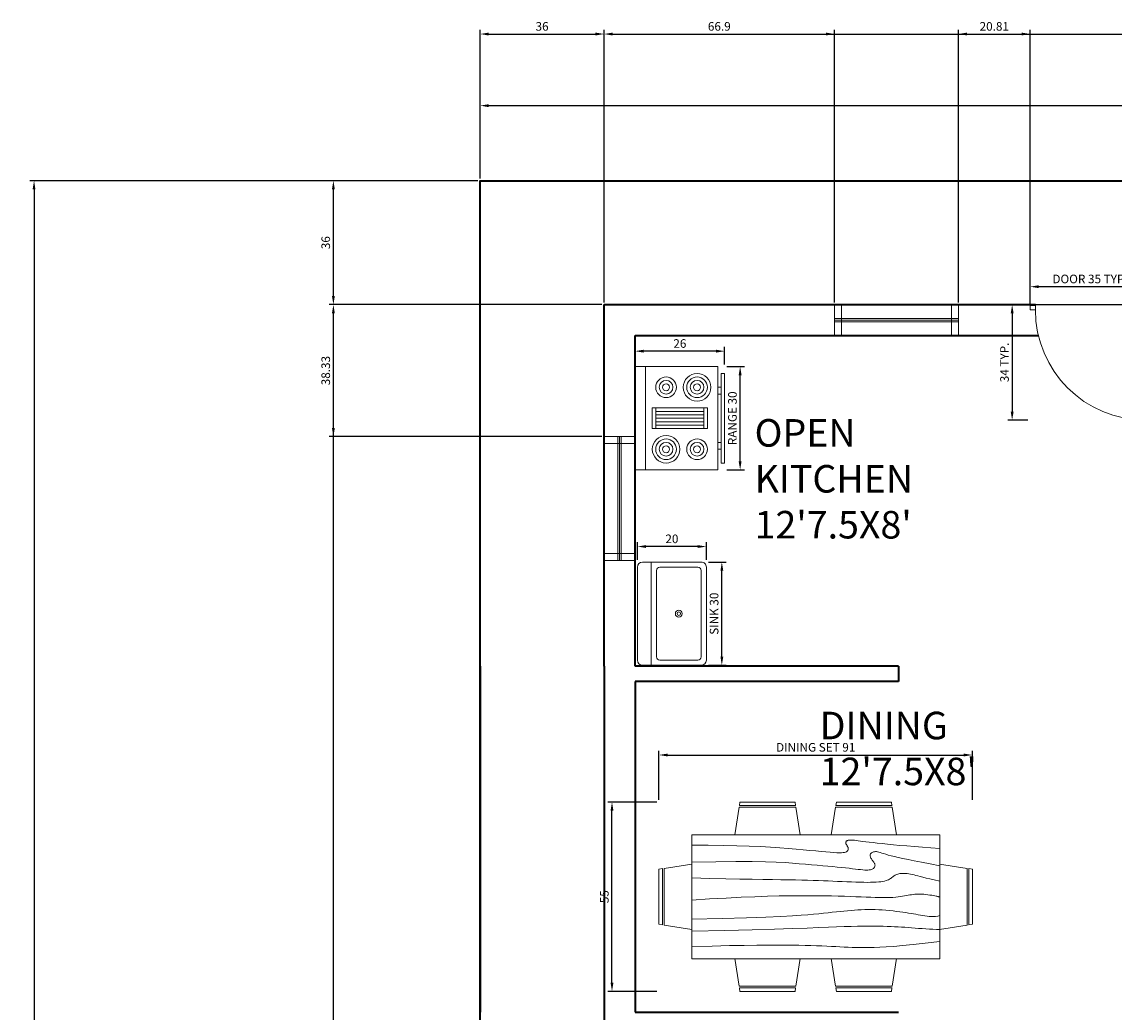
# Model space of a CAD drawing. Units: inches. Extents: x 204 to 942, y 1794 to 2670.
# Tile 4 of 6: x 204 to 521, y 2383 to 2670. Entities that reach past the tile are written whole.
import ezdxf

# ---------------------------------------------------------------- set-up
doc = ezdxf.new("R2010")
doc.units = ezdxf.units.IN
for name, color, linetype, lineweight in [('A-ANNO-DIMS', 2, 'Continuous', 18), ('A-AREA-IDEN', 7, 'Continuous', 18), ('A-DOOR', 3, 'Continuous', 18), ('A-EQPM', 9, 'Continuous', 18), ('A-FLOR-FIXT', 9, 'Continuous', 18), ('A-FLOR-OTLN', 7, 'Continuous', 25), ('A-FURN', 8, 'Continuous', 18), ('A-GLAZ', 4, 'Continuous', 18), ('A-WALL', 7, 'Continuous', 35), ('C-PROP', 7, 'Continuous', 35)]:
    doc.layers.add(name, color=color, linetype=linetype, lineweight=lineweight)
doc.styles.get("Standard").update_dxf_attribs({"font": 'arial.ttf'})
doc.dimstyles.new('ISO-25', dxfattribs={"dimtxt": 2.5, "dimasz": 2.5, "dimexe": 1.25, "dimexo": 0.625, "dimtad": 1, "dimtxsty": 'Standard', "dimcen": 2.5, "dimadec": 0, "dimazin": 0, "dimtfac": 1, "dimtmove": 0, "dimatfit": 3, "dimfxl": 1, "dimarcsym": 0})

# ---------------------------------------------------------------- blocks, each defined once
blk = doc.blocks.new('Dining Set - 36 x 72 in.')
for p, q in [((-22.2343, 26.00059), (-23.4847, 17.99762)), ((-22.2304, 26), (-5.7608, 26)), ((-22, 27.5), (-22.1562, 26.50042)), ((-5.8416, 26.5), (-22.1534, 26.5)), ((-22, 27.5), (-6, 27.5)), ((-5.8437, 26.49966), (-6, 27.5)), ((-4.5152, 17.99762), (-5.7655, 25.99926)), ((5.7657, 26.00059), (4.5153, 17.99762)), ((5.7696, 26), (22.2392, 26)), ((6, 27.5), (5.8438, 26.50042)), ((22.1584, 26.5), (5.8466, 26.5)), ((6, 27.5), (22, 27.5)), ((22.1563, 26.49966), (22, 27.5)), ((23.4848, 17.99762), (22.2345, 25.99926)), ((36, 18), (-36, 18)), ((-36, 18), (-36, -18)), ((36, -18), (36, 18)), ((-45.5, 8), (-44.5004, 8.15617)), ((-45.5, 8), (-45.5, -8)), ((-44.5, -8.15843), (-44.5, 8.15338)), ((-44.0006, 8.23428), (-35.9976, 9.48474)), ((-44, 8.23041), (-44, -8.23915)), ((44.0006, 8.23428), (35.9976, 9.48474)), ((44, 8.23041), (44, -8.23915)), ((44.5, -8.15843), (44.5, 8.15338)), ((45.5, 8), (44.5005, 8.15617)), ((45.5, 8), (45.5, -8)), ((-44.4997, -8.15631), (-45.5, -8)), ((-35.9976, -9.48476), (-43.9993, -8.2345)), ((35.9976, -9.48476), (43.9993, -8.2345)), ((44.4997, -8.15631), (45.5, -8)), ((-36, -18), (36, -18)), ((-22.2343, -26.0006), (-23.4847, -17.99762)), ((-4.5152, -17.99762), (-5.7655, -25.99928)), ((5.7657, -26.0006), (4.5153, -17.99762)), ((23.4848, -17.99762), (22.2345, -25.99928)), ((-22.2304, -26), (-5.7608, -26)), ((-22, -27.5), (-22.1562, -26.50044)), ((-5.8416, -26.5), (-22.1534, -26.5)), ((-22, -27.5), (-6, -27.5)), ((-5.8437, -26.49967), (-6, -27.5)), ((5.7696, -26), (22.2392, -26)), ((6, -27.5), (5.8438, -26.50044)), ((22.1584, -26.5), (5.8466, -26.5)), ((6, -27.5), (22, -27.5)), ((22.1563, -26.49967), (22, -27.5))]:
    blk.add_line(p, q)
for points in [[(-36, 15), (-31.1772, 14.97754), (-26.8079, 14.91406), (-22.8538, 14.81543), (-19.276, 14.6875), (-16.0362, 14.53613), (-13.0957, 14.36718), (-10.4159, 14.18652), (-7.9583, 14), (-5.6904, 13.81315), (-3.6035, 13.63021), (-1.6954, 13.45508), (0.0365, 13.29166), (1.5945, 13.14388), (2.9811, 13.01562), (4.1988, 12.9108), (5.25, 12.83333), (6.1393, 12.78613), (6.8802, 12.76823), (7.4883, 12.77767), (7.9792, 12.8125), (8.3685, 12.87077), (8.6719, 12.95052), (8.9049, 13.0498), (9.0833, 13.16666), (9.2205, 13.29899), (9.3216, 13.44401), (9.3895, 13.59879), (9.4271, 13.76041), (9.4373, 13.92594), (9.4232, 14.09245), (9.3875, 14.257), (9.3333, 14.41666), (9.2638, 14.56917), (9.1836, 14.71484), (9.0975, 14.85465), (9.0104, 14.98958), (8.9272, 15.1206), (8.8529, 15.2487), (8.7922, 15.37483), (8.75, 15.5), (8.7305, 15.62467), (8.7344, 15.74739), (8.7617, 15.86621), (8.8125, 15.97916), (8.8867, 16.08431), (8.9844, 16.17968), (9.1055, 16.26334), (9.25, 16.33333), (9.4189, 16.38802), (9.6172, 16.42708), (9.8506, 16.45052), (10.125, 16.45833), (10.4463, 16.45052), (10.8203, 16.42708), (11.2529, 16.38802), (11.75, 16.33333), (12.3184, 16.26318), (12.9694, 16.17838), (13.7151, 16.07991), (14.5677, 15.96875), (15.5395, 15.84586), (16.6426, 15.71224), (17.8893, 15.56884), (19.2917, 15.41666), (20.859, 15.25667), (22.5879, 15.08984), (24.4721, 14.91715), (26.5052, 14.73958), (28.6809, 14.5581), (30.9929, 14.3737), (33.4347, 14.18733), (36, 14)], [(-36, 10), (-28.9766, 10.14274), (-23.1725, 10.20442), (-18.4241, 10.19775), (-14.5677, 10.13541), (-11.4399, 10.03011), (-8.877, 9.89453), (-6.7154, 9.74137), (-4.7917, 9.58333), (-2.9698, 9.43082), (-1.2246, 9.28515), (0.4415, 9.14534), (2.026, 9.01041), (3.5266, 8.87939), (4.9408, 8.7513), (6.266, 8.62516), (7.5, 8.5), (8.6411, 8.37549), (9.6914, 8.2539), (10.6538, 8.13818), (11.5312, 8.03125), (12.3267, 7.93603), (13.043, 7.85547), (13.6831, 7.79248), (14.25, 7.75), (14.7471, 7.7303), (15.1797, 7.73307), (15.5537, 7.75732), (15.875, 7.80208), (16.1494, 7.86637), (16.3828, 7.94922), (16.5811, 8.04964), (16.75, 8.16666), (16.8944, 8.29915), (17.0143, 8.44531), (17.1089, 8.60319), (17.1771, 8.77083), (17.218, 8.94629), (17.2305, 9.1276), (17.2137, 9.31282), (17.1667, 9.5), (17.0895, 9.6875), (16.987, 9.875), (16.8649, 10.0625), (16.7292, 10.25), (16.5856, 10.4375), (16.4401, 10.625), (16.2985, 10.8125), (16.1667, 11), (16.05, 11.18733), (15.9518, 11.3737), (15.8752, 11.5581), (15.8229, 11.73958), (15.798, 11.91715), (15.8034, 12.08984), (15.842, 12.25667), (15.9167, 12.41666), (16.0295, 12.56836), (16.1784, 12.70833), (16.3605, 12.83268), (16.5729, 12.9375), (16.8127, 13.01888), (17.0768, 13.07291), (17.3625, 13.0957), (17.6667, 13.08333), (17.9894, 13.03312), (18.3418, 12.94726), (18.7382, 12.82918), (19.1927, 12.68229), (19.7195, 12.51001), (20.3327, 12.31575), (21.0465, 12.10294), (21.875, 11.875), (22.8357, 11.63354), (23.959, 11.37304), (25.2786, 11.08618), (26.8282, 10.76562), (28.6414, 10.40405), (30.752, 9.99414), (33.1936, 9.52856), (36, 9)], [(-36, 5.5), (-30.7157, 5.3348), (-26.069, 5.20963), (-21.9946, 5.11767), (-18.4271, 5.05208), (-15.3009, 5.00602), (-12.5508, 4.97265), (-10.1112, 4.94515), (-7.9167, 4.91666), (-5.909, 4.88167), (-4.0586, 4.83984), (-2.3429, 4.79215), (-0.7396, 4.73958), (0.7739, 4.6831), (2.22, 4.6237), (3.6213, 4.56233), (5, 4.5), (6.373, 4.43782), (7.7344, 4.3776), (9.0723, 4.32129), (10.375, 4.27083), (11.6309, 4.22819), (12.8281, 4.19531), (13.9551, 4.17415), (15, 4.16666), (15.954, 4.17448), (16.819, 4.19791), (17.6001, 4.23698), (18.3021, 4.29166), (18.9299, 4.36198), (19.4883, 4.44791), (19.9823, 4.54948), (20.4167, 4.66666), (20.7969, 4.79899), (21.1302, 4.94401), (21.4245, 5.09879), (21.6875, 5.26041), (21.9271, 5.42594), (22.1511, 5.59245), (22.3672, 5.757), (22.5834, 5.91666), (22.8065, 6.06868), (23.0404, 6.21093), (23.2879, 6.34147), (23.5521, 6.45833), (23.8358, 6.55957), (24.142, 6.64323), (24.4735, 6.70735), (24.8334, 6.75), (25.2235, 6.76969), (25.642, 6.76692), (26.0858, 6.74267), (26.5521, 6.69791), (27.0379, 6.63362), (27.5404, 6.55078), (28.0565, 6.45036), (28.5834, 6.33333), (29.1242, 6.19987), (29.7071, 6.04687), (30.3661, 5.87044), (31.1354, 5.66666), (32.0493, 5.43164), (33.142, 5.16146), (34.4475, 4.85221), (36, 4.5)], [(-36, -1), (-30.7915, -0.6591), (-26.0195, -0.38216), (-21.6519, -0.16284), (-17.6563, 0.00521), (-14.0005, 0.12833), (-10.6523, 0.21289), (-7.5796, 0.26522), (-4.75, 0.29166), (-2.134, 0.29793), (0.2878, 0.28711), (2.5317, 0.26163), (4.6146, 0.22396), (6.5529, 0.17651), (8.3633, 0.12174), (10.0623, 0.06209), (11.6667, 0), (13.1899, -0.06201), (14.6341, -0.1211), (15.9982, -0.17432), (17.2813, -0.21875), (18.4823, -0.25147), (19.6003, -0.26953), (20.6343, -0.27002), (21.5834, -0.25), (22.4481, -0.20768), (23.2357, -0.14584), (23.9549, -0.06836), (24.6146, 0.02083), (25.2235, 0.11784), (25.7904, 0.21875), (26.3241, 0.31966), (26.8334, 0.41666), (27.3265, 0.50618), (27.8099, 0.58593), (28.2894, 0.65397), (28.7709, 0.70833), (29.2601, 0.74707), (29.763, 0.76823), (30.2855, 0.76985), (30.8334, 0.75), (31.4088, 0.70784), (31.9994, 0.64713), (32.589, 0.57275), (33.1615, 0.48958), (33.7008, 0.4025), (34.1908, 0.3164), (34.6153, 0.23616), (34.9584, 0.16666), (35.2099, 0.11165), (35.3848, 0.07031), (35.504, 0.04069), (35.5886, 0.02083), (35.6594, 0.00879), (35.7377, 0.0026), (35.8442, 0.00032), (36, 0)], [(-36, -6.5), (-27.1843, -6.31267), (-20.084, -6.1263), (-14.469, -5.9419), (-10.1094, -5.76042), (-6.7752, -5.58285), (-4.2363, -5.41016), (-2.2629, -5.24333), (-0.625, -5.08334), (0.8708, -4.93099), (2.2715, -4.78646), (3.5872, -4.64974), (4.8281, -4.52084), (6.0046, -4.39974), (7.127, -4.28646), (8.2053, -4.18099), (9.25, -4.08334), (10.2705, -3.99382), (11.2734, -3.91407), (12.2647, -3.84603), (13.25, -3.79167), (14.2354, -3.75293), (15.2266, -3.73177), (16.2295, -3.73015), (17.25, -3.75), (18.2912, -3.79248), (19.3451, -3.85547), (20.4009, -3.93604), (21.4479, -4.03125), (22.4754, -4.13819), (23.4727, -4.25391), (24.4289, -4.37549), (25.3334, -4.5), (26.1785, -4.62492), (26.9694, -4.74935), (27.7145, -4.87281), (28.4219, -4.99479), (29.1, -5.11483), (29.7572, -5.23242), (30.4016, -5.34709), (31.0417, -5.45834), (31.6837, -5.56437), (32.3262, -5.65821), (32.9658, -5.73153), (33.599, -5.77604), (34.2224, -5.78345), (34.8327, -5.74545), (35.4264, -5.65373), (36, -5.5)], [(-36, -10), (-26.4022, -9.81299), (-18.4675, -9.62891), (-11.9839, -9.45069), (-6.7396, -9.28125), (-2.5226, -9.12354), (0.8789, -8.98047), (3.6769, -8.85498), (6.0833, -8.75), (8.2767, -8.66765), (10.3021, -8.60677), (12.1712, -8.56543), (13.8958, -8.54167), (15.4876, -8.53353), (16.9583, -8.53907), (18.3197, -8.55632), (19.5834, -8.58334), (20.7616, -8.61841), (21.8685, -8.66081), (22.9188, -8.71004), (23.9271, -8.76563), (24.9081, -8.82707), (25.8763, -8.89388), (26.8465, -8.96558), (27.8334, -9.04167), (28.8474, -9.12118), (29.8828, -9.20117), (30.93, -9.27824), (31.9792, -9.34896), (33.0205, -9.40991), (34.0443, -9.45768), (35.0407, -9.48885), (36, -9.5)], [(-36, -14.5), (-30.0881, -14.33513), (-25.0332, -14.21224), (-20.7312, -14.12647), (-17.0781, -14.07292), (-13.97, -14.04671), (-11.3027, -14.04297), (-8.9724, -14.05681), (-6.875, -14.08334), (-4.9224, -14.11833), (-3.0905, -14.16016), (-1.3709, -14.20785), (0.2448, -14.26042), (1.7647, -14.3169), (3.1973, -14.3763), (4.5507, -14.43767), (5.8333, -14.5), (7.0554, -14.5621), (8.235, -14.62175), (9.3922, -14.67652), (10.5469, -14.72396), (11.7192, -14.76164), (12.929, -14.78711), (14.1965, -14.79794), (15.5417, -14.79167), (16.9933, -14.76424), (18.6152, -14.70508), (20.4804, -14.60197), (22.6615, -14.44271), (25.2312, -14.21509), (28.2624, -13.9069), (31.8277, -13.50594), (36, -13)]]:
    blk.add_lwpolyline(points)
blk = doc.blocks.new('Sink-single - 30 in top')
blk.add_line((-15, -3.999996), (15, -3.999996))
for points in [[(-13.5, 0), (13.5, 0)], [(-15, -18.499996), (-15, -1.5)], [(15, -1.5), (15, -18.499996)], [(-12.5, -5.499996), (12.5, -5.499996)], [(-13.5, -17.499996), (-13.5, -6.499996)], [(13.5, -6.499996), (13.5, -17.499996)], [(12.5, -18.499996), (-12.5, -18.499996)], [(13.5, -19.999996), (-13.5, -19.999996)]]:
    blk.add_lwpolyline(points)
for radius in [1, 0.5]:
    blk.add_circle((0, -11.999996), radius)
for centre, radius, start, end in [((-13.5, -1.5), 1.5, 90, 180), ((13.5, -1.5), 1.5, 0, 90), ((-12.5, -6.499996), 1, 90, 180), ((12.5, -6.499996), 1, 0, 90), ((-13.5, -18.499996), 1.5, 180, 270), ((-12.5, -17.499996), 1, 180, 270), ((12.5, -17.499996), 1, 270, 0), ((13.5, -18.499996), 1.5, 270, 0)]:
    blk.add_arc(centre, radius, start, end)
blk = doc.blocks.new('Range-Oven - 30 in top')
for p, q in [((0, -3), (30, -3)), ((12, -6), (18, -6)), ((13, -20), (13, -6)), ((14, -6), (14, -20)), ((15, -20), (15, -6)), ((16, -6), (16, -20)), ((17, -20), (17, -6)), ((18, -20), (12, -20)), ((6, -24), (6, -25)), ((8, -25), (8, -24)), ((22, -25), (22, -24)), ((24, -24), (24, -25))]:
    blk.add_line(p, q)
for points in [[(0, -24), (0, 0), (30, 0), (30, -24)], [(12, -21), (12, -5), (18, -5), (18, -21)], [(2, -26), (2, -25), (28, -25), (28, -26)]]:
    blk.add_lwpolyline(points, close=True)
for centre, radius in [((6, -9), 4), ((6, -9), 3), ((24, -9), 3), ((6, -9), 2), ((6, -9), 1), ((24, -9), 2), ((24, -9), 1), ((6, -18), 3), ((24, -18), 4), ((24, -18), 3), ((6, -18), 2), ((6, -18), 1), ((24, -18), 2), ((24, -18), 1)]:
    blk.add_circle(centre, radius)
blk = doc.blocks.new('*D10')
at = {"layer": 'A-ANNO-DIMS', "color": 0, "lineweight": -2, "transparency": 16777216}
for p, q in [((336.74, 2624.88), (336.74, 2647.31)), ((339.24, 2646.06), (724.24, 2646.06)), ((726.74, 2624.88), (726.74, 2647.31))]:
    blk.add_line(p, q, dxfattribs=at)
at = {"layer": 'A-ANNO-DIMS', "color": 0, "transparency": 16777216}
for points in [[(339.24, 2646.47), (339.24, 2645.64), (336.74, 2646.06)], [(724.24, 2646.47), (724.24, 2645.64), (726.74, 2646.06)]]:
    blk.add_solid(points, dxfattribs=at)
at = {"layer": 'Defpoints', "color": 0, "transparency": 16777216}
for p in [(726.74, 2646.06), (336.74, 2624.26), (726.74, 2624.26)]:
    blk.add_point(p, dxfattribs=at)
at = {"layer": 'A-ANNO-DIMS', "color": 0, "transparency": 16777216, "insert": (531.74, 2647.96), "char_height": 2.5, "attachment_point": 5}
blk.add_mtext('390', dxfattribs=at)
blk = doc.blocks.new('*D11')
at = {"layer": 'A-ANNO-DIMS', "color": 0, "lineweight": -2, "transparency": 16777216}
for p, q in [((336.12, 2624.26), (205.97, 2624.26)), ((207.22, 2621.76), (207.22, 1840.76)), ((336.12, 1838.26), (205.97, 1838.26))]:
    blk.add_line(p, q, dxfattribs=at)
at = {"layer": 'A-ANNO-DIMS', "color": 0, "transparency": 16777216}
for points in [[(206.8, 2621.76), (207.63, 2621.76), (207.22, 2624.26)], [(206.8, 1840.76), (207.63, 1840.76), (207.22, 1838.26)]]:
    blk.add_solid(points, dxfattribs=at)
at = {"layer": 'Defpoints', "color": 0, "transparency": 16777216}
for p in [(336.74, 2624.26), (207.22, 1838.26), (336.74, 1838.26)]:
    blk.add_point(p, dxfattribs=at)
at = {"layer": 'A-ANNO-DIMS', "color": 0, "transparency": 16777216, "insert": (205.32, 2231.26), "char_height": 2.5, "attachment_point": 5, "rotation": 90}
blk.add_mtext('786', dxfattribs=at)
blk = doc.blocks.new('WIN-36IN')
for p, q in [((0, 9), (36, 9)), ((0, 0), (0, 9)), ((2, 0), (2, 9)), ((34, 0), (34, 9)), ((36, 9), (36, 0)), ((0, 5), (36, 5)), ((0, 4.5), (36, 4.5)), ((0, 4), (36, 4)), ((36, 0), (0, 0)), ((0, 0), (2, 0)), ((36, 0), (34, 0))]:
    blk.add_line(p, q)
blk = doc.blocks.new('DOOR-SWING-32IN')
for p, q in [((3.26, 1.55), (3.26, 33.49)), ((1.26, 1.55), (3.26, 1.55))]:
    blk.add_line(p, q)
blk.add_lwpolyline([(1.26, 33.55), (1.26, 1.55), (3.26, 1.55)])
for points in [[(1.26, 1.55), (0, 1.55), (0, 0), (1.26, 0)], [(33.26, 1.55), (34.79, 1.55), (34.79, 0.26), (33.26, 0.26)]]:
    blk.add_lwpolyline(points, close=True)
blk.add_arc((1.26, 1.55), 32, 0, 90)
blk = doc.blocks.new('*D16')
at = {"layer": 'A-ANNO-DIMS', "color": 0, "lineweight": -2, "transparency": 16777216}
for p, q in [((496.46, 2588.88), (496.46, 2594.73)), ((531.24, 2588.88), (531.24, 2594.73)), ((528.74, 2593.48), (498.96, 2593.48))]:
    blk.add_line(p, q, dxfattribs=at)
at = {"layer": 'A-ANNO-DIMS', "color": 0, "transparency": 16777216}
for points in [[(498.96, 2593.89), (498.96, 2593.06), (496.46, 2593.48)], [(528.74, 2593.89), (528.74, 2593.06), (531.24, 2593.48)]]:
    blk.add_solid(points, dxfattribs=at)
at = {"layer": 'Defpoints', "color": 0, "transparency": 16777216}
for p in [(496.46, 2593.48), (496.46, 2588.26), (531.24, 2588.26)]:
    blk.add_point(p, dxfattribs=at)
at = {"layer": 'A-ANNO-DIMS', "color": 0, "transparency": 16777216, "insert": (513.85, 2595.4), "char_height": 2.5, "attachment_point": 5}
blk.add_mtext('DOOR 35 TYP.', dxfattribs=at)
blk = doc.blocks.new('*D17')
at = {"layer": 'A-ANNO-DIMS', "color": 0, "lineweight": -2, "transparency": 16777216}
for p, q in [((495.83, 2588.26), (489.99, 2588.26)), ((491.24, 2585.76), (491.24, 2557.21)), ((495.83, 2554.71), (489.99, 2554.71))]:
    blk.add_line(p, q, dxfattribs=at)
at = {"layer": 'A-ANNO-DIMS', "color": 0, "transparency": 16777216}
for points in [[(490.82, 2585.76), (491.66, 2585.76), (491.24, 2588.26)], [(490.82, 2557.21), (491.66, 2557.21), (491.24, 2554.71)]]:
    blk.add_solid(points, dxfattribs=at)
at = {"layer": 'Defpoints', "color": 0, "transparency": 16777216}
for p in [(496.46, 2588.26), (491.24, 2554.71), (496.46, 2554.71)]:
    blk.add_point(p, dxfattribs=at)
at = {"layer": 'A-ANNO-DIMS', "color": 0, "transparency": 16777216, "insert": (489.34, 2571.48), "char_height": 2.5, "attachment_point": 5, "rotation": 90}
blk.add_mtext('34 TYP.', dxfattribs=at)
blk = doc.blocks.new('*D28')
at = {"layer": 'A-ANNO-DIMS', "color": 0, "lineweight": -2, "transparency": 16777216}
for p, q in [((388.69, 2444.42), (388.69, 2458.7)), ((479.69, 2444.42), (479.69, 2458.7)), ((391.19, 2457.45), (477.19, 2457.45))]:
    blk.add_line(p, q, dxfattribs=at)
at = {"layer": 'A-ANNO-DIMS', "color": 0, "transparency": 16777216}
for points in [[(391.19, 2457.86), (391.19, 2457.03), (388.69, 2457.45)], [(477.19, 2457.86), (477.19, 2457.03), (479.69, 2457.45)]]:
    blk.add_solid(points, dxfattribs=at)
at = {"layer": 'Defpoints', "color": 0, "transparency": 16777216}
for p in [(479.69, 2457.45), (388.69, 2443.8), (479.69, 2443.8)]:
    blk.add_point(p, dxfattribs=at)
at = {"layer": 'A-ANNO-DIMS', "color": 0, "transparency": 16777216, "insert": (434.19, 2459.36), "char_height": 2.5, "attachment_point": 5}
blk.add_mtext('DINING SET 91', dxfattribs=at)
blk = doc.blocks.new('*D29')
at = {"layer": 'A-ANNO-DIMS', "color": 0, "lineweight": -2, "transparency": 16777216}
for p, q in [((388.07, 2443.8), (373.79, 2443.8)), ((375.04, 2391.3), (375.04, 2441.3)), ((388.07, 2388.8), (373.79, 2388.8))]:
    blk.add_line(p, q, dxfattribs=at)
at = {"layer": 'A-ANNO-DIMS', "color": 0, "transparency": 16777216}
for points in [[(374.62, 2441.3), (375.46, 2441.3), (375.04, 2443.8)], [(374.62, 2391.3), (375.46, 2391.3), (375.04, 2388.8)]]:
    blk.add_solid(points, dxfattribs=at)
at = {"layer": 'Defpoints', "color": 0, "transparency": 16777216}
for p in [(375.04, 2443.8), (388.69, 2443.8), (388.69, 2388.8)]:
    blk.add_point(p, dxfattribs=at)
at = {"layer": 'A-ANNO-DIMS', "color": 0, "transparency": 16777216, "insert": (373.14, 2416.3), "char_height": 2.5, "attachment_point": 5, "rotation": 90}
blk.add_mtext('55', dxfattribs=at)
blk = doc.blocks.new('*D30')
at = {"layer": 'A-ANNO-DIMS', "color": 0, "lineweight": -2, "transparency": 16777216}
for p, q in [((403.07, 2513.5), (408.19, 2513.5)), ((406.94, 2486), (406.94, 2511)), ((403.07, 2483.5), (408.19, 2483.5))]:
    blk.add_line(p, q, dxfattribs=at)
at = {"layer": 'A-ANNO-DIMS', "color": 0, "transparency": 16777216}
for points in [[(406.53, 2511), (407.36, 2511), (406.94, 2513.5)], [(406.53, 2486), (407.36, 2486), (406.94, 2483.5)]]:
    blk.add_solid(points, dxfattribs=at)
at = {"layer": 'Defpoints', "color": 0, "transparency": 16777216}
for p in [(402.44, 2513.5), (406.94, 2513.5), (402.44, 2483.5)]:
    blk.add_point(p, dxfattribs=at)
at = {"layer": 'A-ANNO-DIMS', "color": 0, "transparency": 16777216, "insert": (405.02, 2498.5), "char_height": 2.5, "attachment_point": 5, "rotation": 90}
blk.add_mtext('SINK 30', dxfattribs=at)
blk = doc.blocks.new('*D31')
at = {"layer": 'A-ANNO-DIMS', "color": 0, "lineweight": -2, "transparency": 16777216}
for p, q in [((382.44, 2514.13), (382.44, 2519.25)), ((402.44, 2514.13), (402.44, 2519.25)), ((399.94, 2518), (384.94, 2518))]:
    blk.add_line(p, q, dxfattribs=at)
at = {"layer": 'A-ANNO-DIMS', "color": 0, "transparency": 16777216}
for points in [[(384.94, 2518.42), (384.94, 2517.59), (382.44, 2518)], [(399.94, 2518.42), (399.94, 2517.59), (402.44, 2518)]]:
    blk.add_solid(points, dxfattribs=at)
at = {"layer": 'Defpoints', "color": 0, "transparency": 16777216}
for p in [(382.44, 2518), (382.44, 2513.5), (402.44, 2513.5)]:
    blk.add_point(p, dxfattribs=at)
at = {"layer": 'A-ANNO-DIMS', "color": 0, "transparency": 16777216, "insert": (392.44, 2519.91), "char_height": 2.5, "attachment_point": 5}
blk.add_mtext('20', dxfattribs=at)
blk = doc.blocks.new('*D32')
at = {"layer": 'A-ANNO-DIMS', "color": 0, "lineweight": -2, "transparency": 16777216}
for p, q in [((408.37, 2570.25), (413.5, 2570.25)), ((412.25, 2542.75), (412.25, 2567.75)), ((408.37, 2540.25), (413.5, 2540.25))]:
    blk.add_line(p, q, dxfattribs=at)
at = {"layer": 'A-ANNO-DIMS', "color": 0, "transparency": 16777216}
for points in [[(411.83, 2567.75), (412.67, 2567.75), (412.25, 2570.25)], [(411.83, 2542.75), (412.67, 2542.75), (412.25, 2540.25)]]:
    blk.add_solid(points, dxfattribs=at)
at = {"layer": 'Defpoints', "color": 0, "transparency": 16777216}
for p in [(407.75, 2570.25), (412.25, 2570.25), (407.75, 2540.25)]:
    blk.add_point(p, dxfattribs=at)
at = {"layer": 'A-ANNO-DIMS', "color": 0, "transparency": 16777216, "insert": (410.33, 2555.25), "char_height": 2.5, "attachment_point": 5, "rotation": 90}
blk.add_mtext('RANGE 30', dxfattribs=at)
blk = doc.blocks.new('*D33')
at = {"layer": 'A-ANNO-DIMS', "color": 0, "lineweight": -2, "transparency": 16777216}
for p, q in [((381.75, 2570.87), (381.75, 2576)), ((407.75, 2570.87), (407.75, 2576)), ((405.25, 2574.75), (384.25, 2574.75))]:
    blk.add_line(p, q, dxfattribs=at)
at = {"layer": 'A-ANNO-DIMS', "color": 0, "transparency": 16777216}
for points in [[(384.25, 2575.17), (384.25, 2574.33), (381.75, 2574.75)], [(405.25, 2575.17), (405.25, 2574.33), (407.75, 2574.75)]]:
    blk.add_solid(points, dxfattribs=at)
at = {"layer": 'Defpoints', "color": 0, "transparency": 16777216}
for p in [(381.75, 2574.75), (381.75, 2570.25), (407.75, 2570.25)]:
    blk.add_point(p, dxfattribs=at)
at = {"layer": 'A-ANNO-DIMS', "color": 0, "transparency": 16777216, "insert": (394.75, 2576.65), "char_height": 2.5, "attachment_point": 5}
blk.add_mtext('26', dxfattribs=at)
blk = doc.blocks.new('*D38')
at = {"layer": 'A-ANNO-DIMS', "color": 0, "lineweight": -2, "transparency": 16777216}
for p, q in [((372.74, 2624.88), (372.74, 2668.11)), ((690.74, 2624.88), (690.74, 2668.11)), ((375.24, 2666.86), (688.24, 2666.86))]:
    blk.add_line(p, q, dxfattribs=at)
at = {"layer": 'A-ANNO-DIMS', "color": 0, "transparency": 16777216}
for points in [[(375.24, 2667.28), (375.24, 2666.44), (372.74, 2666.86)], [(688.24, 2667.28), (688.24, 2666.44), (690.74, 2666.86)]]:
    blk.add_solid(points, dxfattribs=at)
at = {"layer": 'Defpoints', "color": 0, "transparency": 16777216}
for p in [(690.74, 2666.86), (372.74, 2624.26), (690.74, 2624.26)]:
    blk.add_point(p, dxfattribs=at)
at = {"layer": 'A-ANNO-DIMS', "color": 0, "transparency": 16777216, "insert": (531.74, 2668.76), "char_height": 2.5, "attachment_point": 5}
blk.add_mtext('318', dxfattribs=at)
blk = doc.blocks.new('*D39')
at = {"layer": 'A-ANNO-DIMS', "color": 0, "lineweight": -2, "transparency": 16777216}
for p, q in [((372.12, 2588.26), (292.89, 2588.26)), ((294.14, 2140.76), (294.14, 2585.76)), ((336.12, 2138.26), (292.89, 2138.26))]:
    blk.add_line(p, q, dxfattribs=at)
at = {"layer": 'A-ANNO-DIMS', "color": 0, "transparency": 16777216}
for points in [[(293.73, 2585.76), (294.56, 2585.76), (294.14, 2588.26)], [(293.73, 2140.76), (294.56, 2140.76), (294.14, 2138.26)]]:
    blk.add_solid(points, dxfattribs=at)
at = {"layer": 'Defpoints', "color": 0, "transparency": 16777216}
for p in [(294.14, 2588.26), (372.74, 2588.26), (336.74, 2138.26)]:
    blk.add_point(p, dxfattribs=at)
at = {"layer": 'A-ANNO-DIMS', "color": 0, "transparency": 16777216, "insert": (292.24, 2363.26), "char_height": 2.5, "attachment_point": 5, "rotation": 90}
blk.add_mtext('450', dxfattribs=at)
blk = doc.blocks.new('*D40')
at = {"layer": 'A-ANNO-DIMS', "color": 0, "lineweight": -2, "transparency": 16777216}
for p, q in [((336.74, 2624.88), (336.74, 2668.11)), ((372.74, 2588.88), (372.74, 2668.11)), ((339.24, 2666.86), (370.24, 2666.86))]:
    blk.add_line(p, q, dxfattribs=at)
at = {"layer": 'A-ANNO-DIMS', "color": 0, "transparency": 16777216}
for points in [[(339.24, 2667.28), (339.24, 2666.44), (336.74, 2666.86)], [(370.24, 2667.28), (370.24, 2666.44), (372.74, 2666.86)]]:
    blk.add_solid(points, dxfattribs=at)
at = {"layer": 'Defpoints', "color": 0, "transparency": 16777216}
for p in [(372.74, 2666.86), (336.74, 2624.26), (372.74, 2588.26)]:
    blk.add_point(p, dxfattribs=at)
at = {"layer": 'A-ANNO-DIMS', "color": 0, "transparency": 16777216, "insert": (354.74, 2668.76), "char_height": 2.5, "attachment_point": 5}
blk.add_mtext('36', dxfattribs=at)
blk = doc.blocks.new('*D42')
at = {"layer": 'A-ANNO-DIMS', "color": 0, "lineweight": -2, "transparency": 16777216}
for p, q in [((336.12, 2624.26), (292.89, 2624.26)), ((294.14, 2590.76), (294.14, 2621.76)), ((372.12, 2588.26), (292.89, 2588.26))]:
    blk.add_line(p, q, dxfattribs=at)
at = {"layer": 'A-ANNO-DIMS', "color": 0, "transparency": 16777216}
for points in [[(293.73, 2621.76), (294.56, 2621.76), (294.14, 2624.26)], [(293.73, 2590.76), (294.56, 2590.76), (294.14, 2588.26)]]:
    blk.add_solid(points, dxfattribs=at)
at = {"layer": 'Defpoints', "color": 0, "transparency": 16777216}
for p in [(294.14, 2624.26), (336.74, 2624.26), (372.74, 2588.26)]:
    blk.add_point(p, dxfattribs=at)
at = {"layer": 'A-ANNO-DIMS', "color": 0, "transparency": 16777216, "insert": (292.24, 2606.26), "char_height": 2.5, "attachment_point": 5, "rotation": 90}
blk.add_mtext('36', dxfattribs=at)
blk = doc.blocks.new('*D51')
at = {"layer": 'A-ANNO-DIMS', "color": 0, "lineweight": -2, "transparency": 16777216}
for p, q in [((372.74, 2588.88), (372.74, 2668.11)), ((439.65, 2588.91), (439.65, 2668.11)), ((375.24, 2666.86), (437.15, 2666.86))]:
    blk.add_line(p, q, dxfattribs=at)
at = {"layer": 'A-ANNO-DIMS', "color": 0, "transparency": 16777216}
for points in [[(375.24, 2667.28), (375.24, 2666.44), (372.74, 2666.86)], [(437.15, 2667.28), (437.15, 2666.44), (439.65, 2666.86)]]:
    blk.add_solid(points, dxfattribs=at)
at = {"layer": 'Defpoints', "color": 0, "transparency": 16777216}
for p in [(439.65, 2666.86), (372.74, 2588.26), (439.65, 2588.28)]:
    blk.add_point(p, dxfattribs=at)
at = {"layer": 'A-ANNO-DIMS', "color": 0, "transparency": 16777216, "insert": (406.2, 2668.76), "char_height": 2.5, "attachment_point": 5}
blk.add_mtext('66.9', dxfattribs=at)
blk = doc.blocks.new('*D52')
at = {"layer": 'A-ANNO-DIMS', "color": 0, "lineweight": -2, "transparency": 16777216}
for p, q in [((475.65, 2588.91), (475.65, 2668.11)), ((496.46, 2588.63), (496.46, 2668.11)), ((478.15, 2666.86), (493.96, 2666.86))]:
    blk.add_line(p, q, dxfattribs=at)
at = {"layer": 'A-ANNO-DIMS', "color": 0, "transparency": 16777216}
for points in [[(478.15, 2667.28), (478.15, 2666.44), (475.65, 2666.86)], [(493.96, 2667.28), (493.96, 2666.44), (496.46, 2666.86)]]:
    blk.add_solid(points, dxfattribs=at)
at = {"layer": 'Defpoints', "color": 0, "transparency": 16777216}
for p in [(496.46, 2666.86), (475.65, 2588.28), (496.46, 2588)]:
    blk.add_point(p, dxfattribs=at)
at = {"layer": 'A-ANNO-DIMS', "color": 0, "transparency": 16777216, "insert": (486.05, 2668.76), "char_height": 2.5, "attachment_point": 5}
blk.add_mtext('20.81', dxfattribs=at)
blk = doc.blocks.new('*D56')
at = {"layer": 'A-ANNO-DIMS', "color": 0, "lineweight": -2, "transparency": 16777216}
for p, q in [((372.12, 2588.26), (292.89, 2588.26)), ((294.14, 2552.43), (294.14, 2585.76)), ((372.12, 2549.93), (292.89, 2549.93))]:
    blk.add_line(p, q, dxfattribs=at)
at = {"layer": 'A-ANNO-DIMS', "color": 0, "transparency": 16777216}
for points in [[(293.73, 2585.76), (294.56, 2585.76), (294.14, 2588.26)], [(293.73, 2552.43), (294.56, 2552.43), (294.14, 2549.93)]]:
    blk.add_solid(points, dxfattribs=at)
at = {"layer": 'Defpoints', "color": 0, "transparency": 16777216}
for p in [(294.14, 2588.26), (372.74, 2588.26), (372.75, 2549.93)]:
    blk.add_point(p, dxfattribs=at)
at = {"layer": 'A-ANNO-DIMS', "color": 0, "transparency": 16777216, "insert": (292.24, 2569.1), "char_height": 2.5, "attachment_point": 5, "rotation": 90}
blk.add_mtext('38.33', dxfattribs=at)

msp = doc.modelspace()

# ---------------------------------------------------------------- linework, layer by layer
at = {"layer": 'A-FLOR-OTLN'}
msp.add_lwpolyline([(372.7443, 2588.2597), (690.7443, 2588.2597), (690.7443, 2138.2597), (372.7443, 2138.2597)], close=True, dxfattribs=at)
at = {"layer": 'A-WALL'}
for p, q in [((372.7443, 2588.2597), (498.0198, 2588.2597)), ((372.7443, 2483.2597), (372.7443, 2588.2597)), ((381.7443, 2579.2597), (498.8612, 2579.2597)), ((381.7443, 2483.2597), (381.7443, 2579.2597)), ((372.7443, 2483.2597), (372.7443, 2382.7597)), ((458.2443, 2483.2597), (381.7443, 2483.2597)), ((458.2443, 2483.2597), (381.7443, 2483.2597)), ((458.2443, 2483.2597), (458.2443, 2478.7597)), ((458.2443, 2478.7597), (381.7443, 2478.7597)), ((381.7443, 2478.7597), (381.7443, 2382.7597)), ((458.2443, 2478.7597), (381.7443, 2478.7597)), ((458.2443, 2478.7597), (449.3699, 2478.7597)), ((372.7443, 2382.7597), (372.7443, 2325.7597)), ((381.7443, 2382.7597), (458.2443, 2382.7597))]:
    msp.add_line(p, q, dxfattribs=at)
at = {"layer": 'C-PROP'}
for p, q in [((372.7443, 2624.2597), (498.0198, 2624.2597)), ((336.7443, 2483.2597), (336.7443, 2588.2597)), ((336.7443, 2483.2597), (336.7443, 2382.7597))]:
    msp.add_line(p, q, dxfattribs=at)
msp.add_lwpolyline([(336.7443, 2102.2597), (336.7443, 2624.2597), (726.7443, 2624.2597), (726.7443, 2102.2597)], dxfattribs=at)

# ---------------------------------------------------------------- block references
at = {"layer": 'A-DOOR', "rotation": 180}
msp.add_blockref('DOOR-SWING-32IN', (531.2446, 2588.2593), dxfattribs=at)
at = {"layer": 'A-EQPM', "rotation": 90}
msp.add_blockref('Range-Oven - 30 in top', (381.7497, 2540.2494), dxfattribs=at)
at = {"layer": 'A-FLOR-FIXT', "rotation": 90.00000000000006}
msp.add_blockref('Sink-single - 30 in top', (382.4424, 2498.5042), dxfattribs=at)
at = {"layer": 'A-FURN'}
msp.add_blockref('Dining Set - 36 x 72 in.', (434.1904, 2416.2951), dxfattribs=at)
at = {"layer": 'A-GLAZ'}
msp.add_blockref('WIN-36IN', (439.65, 2579.28), dxfattribs=at)
at = {"layer": 'A-GLAZ', "rotation": 269.9999999999983}
msp.add_blockref('WIN-36IN', (372.7495, 2549.9321), dxfattribs=at)

# ---------------------------------------------------------------- texts
at = {"layer": 'A-AREA-IDEN', "char_height": 2.5, "attachment_point": 1}
for s, width, insert in [("{\\H3.2x;OPEN KITCHEN\\P12'7.5X8' }", 46.676204, (416.4456, 2555.0111)), ("{\\H3.2x;DINING\\P12'7.5X8' }", 47.131823, (435.3499, 2470.0165))]:
    msp.add_mtext_dynamic_manual_height_columns(s, width=width, gutter_width=12.5, heights=[0], dxfattribs=dict(at, insert=insert))

# ---------------------------------------------------------------- dimensions: what is measured, and where the dimension line sits
at = {"layer": 'A-ANNO-DIMS'}
for base, p1, p2, override, picture, middle in [((372.7443, 2666.8597), (336.7443, 2624.2597), (372.7443, 2588.2597), {"dimdec": 0, "dimlfac": 1, "dimrnd": 0, "dimzin": 0, "dimdsep": 46, "dimlunit": 2}, '*D40', (354.7443, 2668.7619)), ((690.7443, 2666.8597), (372.7443, 2624.2597), (690.7443, 2624.2597), {"dimdec": 0, "dimlfac": 1, "dimrnd": 0, "dimzin": 0, "dimdsep": 46, "dimlunit": 2}, '*D38', (531.7443, 2668.7619)), ((439.6495, 2666.8597), (372.7443, 2588.2597), (439.6495, 2588.2802), {"dimdec": 1, "dimlfac": 1, "dimrnd": 0, "dimzin": 0, "dimdsep": 46, "dimlunit": 2}, '*D51', (406.1969, 2668.7611)), ((496.4586, 2666.8597), (475.6495, 2588.2802), (496.4586, 2588.0038), {"dimdec": 2, "dimlfac": 1, "dimrnd": 0, "dimzin": 0, "dimdsep": 46, "dimlunit": 2}, '*D52', (486.0541, 2668.7611)), ((726.7443, 2646.0578), (336.7443, 2624.2597), (726.7443, 2624.2597), {"dimclrd": 0, "dimclre": 0, "dimclrt": 0}, '*D10', (531.7443, 2647.9601))]:
    dim = msp.add_linear_dim(base=base, p1=p1, p2=p2, dimstyle='ISO-25', override=override, dxfattribs=at)
    dim.commit()
    dim.dimension.update_dxf_attribs({"geometry": picture, "text_midpoint": middle})
for base, p1, p2, angle, override, picture, middle in [((207.2181, 1838.2597), (336.7443, 2624.2597), (336.7443, 1838.2597), 90, {"dimclrd": 0, "dimclre": 0, "dimclrt": 0}, '*D11', (205.3166, 2231.2597)), ((294.1443, 2624.2597), (372.7443, 2588.2597), (336.7443, 2624.2597), 90, {"dimdec": 0, "dimlfac": 1, "dimrnd": 0, "dimzin": 0, "dimdsep": 46, "dimlunit": 2}, '*D42', (292.242, 2606.2597)), ((294.1443, 2588.2597), (372.7497, 2549.9325), (372.7443, 2588.2597), 90, {"dimdec": 2, "dimlfac": 1, "dimrnd": 0, "dimzin": 0, "dimdsep": 46, "dimlunit": 2}, '*D56', (292.242, 2569.0961)), ((294.1443, 2588.2597), (336.7443, 2138.2597), (372.7443, 2588.2597), 90, {"dimdec": 0, "dimlfac": 1, "dimrnd": 0, "dimzin": 0, "dimdsep": 46, "dimlunit": 2}, '*D39', (292.2429, 2363.2597)), ((381.7497, 2574.7494), (407.7497, 2570.2494), (381.7497, 2570.2494), 180, {"dimdec": 0, "dimlfac": 1, "dimrnd": 0, "dimzin": 0, "dimdsep": 46, "dimlunit": 2}, '*D33', (394.7497, 2576.6509)), ((382.4424, 2518.0042), (402.4424, 2513.5042), (382.4424, 2513.5042), 180, {"dimdec": 0, "dimlfac": 1, "dimrnd": 0, "dimzin": 0, "dimdsep": 46, "dimlunit": 2}, '*D31', (392.4424, 2519.9057)), ((375.0404, 2443.7951), (388.6904, 2388.7951), (388.6904, 2443.7951), 90, {"dimdec": 0, "dimlfac": 1, "dimrnd": 0, "dimzin": 0, "dimdsep": 46, "dimlunit": 2}, '*D29', (373.1441, 2416.2951))]:
    dim = msp.add_linear_dim(base=base, p1=p1, p2=p2, angle=angle, dimstyle='ISO-25', override=override, dxfattribs=at)
    dim.commit()
    dim.dimension.update_dxf_attribs({"geometry": picture, "text_midpoint": middle})
for base, p1, p2, angle, text, picture, middle in [((496.4586, 2593.4775), (531.2443, 2588.2597), (496.4586, 2588.2597), 180, 'DOOR <> TYP.', '*D16', (513.8515, 2595.3969)), ((491.2408, 2554.7082), (496.4586, 2588.2597), (496.4586, 2554.7082), 270, '<> TYP.', '*D17', (489.3385, 2571.4839)), ((412.2497, 2570.2494), (407.7497, 2540.2494), (407.7497, 2570.2494), 90, 'RANGE <>', '*D32', (410.3312, 2555.2494)), ((406.9424, 2513.5042), (402.4424, 2483.5042), (402.4424, 2513.5042), 90, 'SINK <>', '*D30', (405.024, 2498.5042))]:
    dim = msp.add_linear_dim(base=base, p1=p1, p2=p2, angle=angle, text=text, dimstyle='ISO-25', override={"dimdec": 0, "dimlfac": 1, "dimrnd": 0, "dimzin": 0, "dimdsep": 46, "dimlunit": 2}, dxfattribs=at)
    dim.commit()
    dim.dimension.update_dxf_attribs({"geometry": picture, "text_midpoint": middle})
dim = msp.add_linear_dim(base=(479.6904, 2457.4451), p1=(388.6904, 2443.7951), p2=(479.6904, 2443.7951), text='DINING SET <>', dimstyle='ISO-25', override={"dimdec": 0, "dimlfac": 1, "dimrnd": 0, "dimzin": 0, "dimdsep": 46, "dimlunit": 2}, dxfattribs=at)
dim.commit()
dim.dimension.update_dxf_attribs({"geometry": '*D28', "text_midpoint": (434.1904, 2459.3627)})

doc.saveas('drawing.dxf')
